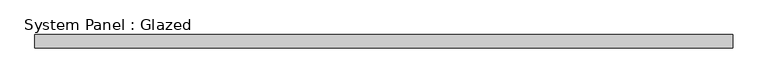
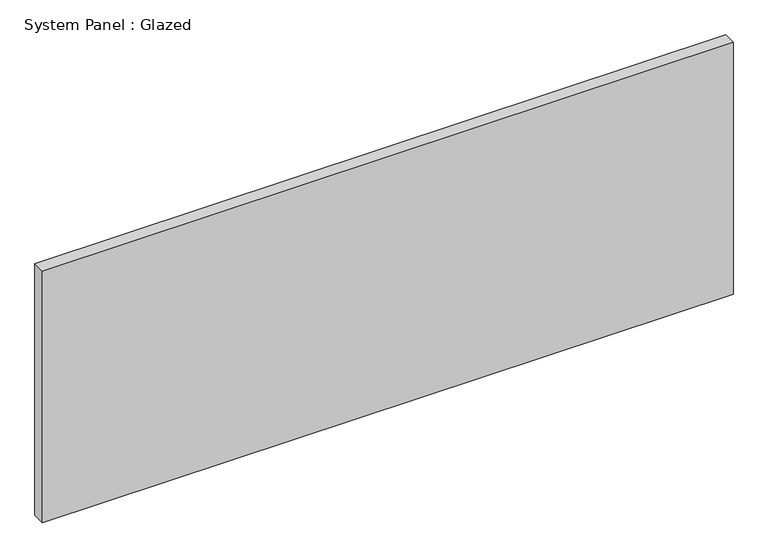
"""IFC4 building model written with IfcOpenShell, lengths in millimetres: plate geometry, System Panel : Glazed."""

from ifc_helpers import new_model, si_unit, origin, origin_with_axes, place, context, project, spatial, polyline, outline, extrude, source, transform, mapped, element, save


def system_panel_glazed_652faff5(model_context):
    return source(origin(), model_context, "Body", "SweptSolid", [
        extrude(outline(polyline([(667.1592567, 19.05), (-667.1592567, 19.05), (-667.1592567, 44.45), (667.1592567, 44.45), (667.1592567, 19.05)])), origin_with_axes(), (0.0, 0.0, 1.0), 514.35),
    ])


if __name__ == "__main__":
    model = new_model("IFC4")
    model_context = context("Model", 3, world=origin())
    ifc_project = project(units=[si_unit("LENGTHUNIT", "METRE", prefix="MILLI")], contexts=[model_context])
    site = spatial("IfcSite", under=ifc_project)
    building = spatial("IfcBuilding", under=site)
    placement = place(None, origin())
    system_panel_glazed_shape = system_panel_glazed_652faff5(model_context)
    element("IfcPlate", 1, ObjectType="System Panel : Glazed", at=placement, inside=building, context=model_context, shape_type="MappedRepresentation", body=[
        mapped(system_panel_glazed_shape, transform((0.0, 0.0, 0.0), x_axis=(1.0, 0.0, 0.0), y_axis=(0.0, 1.0, 0.0), z_axis=(0.0, 0.0, 1.0))),
    ])
    save(model, "model.ifc")

# Revit data of these elements
# Type "System Panel : Glazed"
#   Construction Type Id = "GSP4R"
#   Analytic Construction = "1/8 in Pilkington single glazing"
#   Visual Light Transmittance = 0.9
#   Solar Heat Gain Coefficient = 0.86
#   Heat Transfer Coefficient (U) = 1.18115 BTU/(h·ft²·°F)
# Element 1 (IfcPlate, "System Panel : Glazed")
#   Materials on its faces: "Glass"
# Materials
#   "Glass": class "Glass", colour RGB 0 128 192, transparency 0.75, Description = "Soda Lime Glass", Cost = 0
